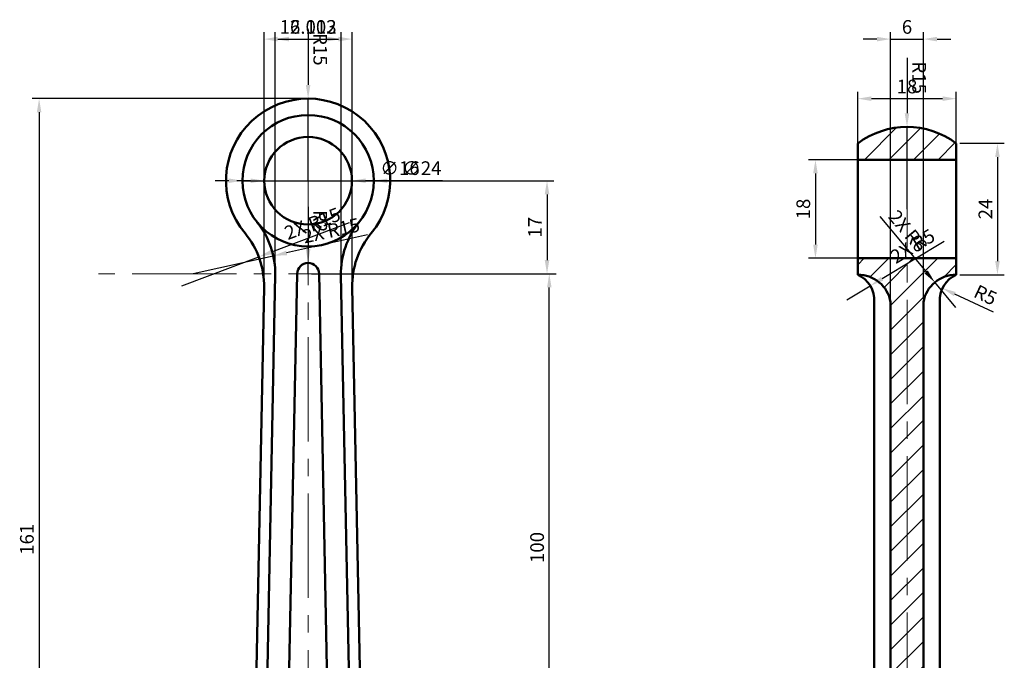
# Model space of a CAD drawing. Units: millimetres. Extents: x 2995 to 3180, y 2734 to 2968.
# Tile 3 of 3: x 2995 to 3175, y 2851 to 2968. Entities that reach past the tile are written whole.
import ezdxf

# ---------------------------------------------------------------- set-up
doc = ezdxf.new("R2010")
doc.units = ezdxf.units.MM
doc.linetypes.add('CENTER2', pattern=[28.575, 19.05, -3.175, 3.175, -3.175])
for name, color, linetype, lineweight in [('M-CNTR', 1, 'CENTER2', 18), ('M-DIMS', 2, 'Continuous', 25), ('M-HATC', 8, 'Continuous', 18), ('M-OUTL', 7, 'Continuous', 50)]:
    doc.layers.add(name, color=color, linetype=linetype, lineweight=lineweight)
doc.styles.get("Standard").update_dxf_attribs({"font": 'arial.ttf'})
doc.dimstyles.new('ISO-25', dxfattribs={"dimtxt": 2.5, "dimasz": 2.5, "dimexe": 1.25, "dimexo": 0.625, "dimtad": 1, "dimtxsty": 'Standard', "dimcen": 2.5, "dimadec": 0, "dimazin": 0, "dimtfac": 1, "dimtmove": 0, "dimatfit": 3, "dimfxl": 1, "dimarcsym": 0})

# ---------------------------------------------------------------- blocks, each defined once
blk = doc.blocks.new('*D15')
at = {"layer": 'Defpoints', "color": 0, "transparency": 16777216}
for p in [(3049.54, 2921.77), (3091.59, 2921.77), (3047.54, 2821.77)]:
    blk.add_point(p, dxfattribs=at)
at = {"layer": 'M-DIMS', "color": 0, "lineweight": -2, "transparency": 16777216}
for p, q in [((3050.17, 2921.77), (3092.84, 2921.77)), ((3091.59, 2824.27), (3091.59, 2919.27)), ((3048.17, 2821.77), (3092.84, 2821.77))]:
    blk.add_line(p, q, dxfattribs=at)
at = {"layer": 'M-DIMS', "color": 0, "transparency": 16777216}
for points in [[(3091.18, 2919.27), (3092.01, 2919.27), (3091.59, 2921.77)], [(3091.18, 2824.27), (3092.01, 2824.27), (3091.59, 2821.77)]]:
    blk.add_solid(points, dxfattribs=at)
at = {"layer": 'M-DIMS', "color": 0, "transparency": 16777216, "insert": (3089.69, 2871.77), "char_height": 2.5, "attachment_point": 5, "rotation": 90}
blk.add_mtext('100', dxfattribs=at)
blk = doc.blocks.new('*D16')
at = {"layer": 'Defpoints', "color": 0, "transparency": 16777216}
for p in [(3047.54, 2938.77), (3047.54, 2921.77), (3091.18, 2921.77)]:
    blk.add_point(p, dxfattribs=at)
at = {"layer": 'M-DIMS', "color": 0, "lineweight": -2, "transparency": 16777216}
for p, q in [((3048.17, 2938.77), (3092.43, 2938.77)), ((3091.18, 2936.27), (3091.18, 2924.27)), ((3048.17, 2921.77), (3092.43, 2921.77))]:
    blk.add_line(p, q, dxfattribs=at)
at = {"layer": 'M-DIMS', "color": 0, "transparency": 16777216}
for points in [[(3090.76, 2936.27), (3091.6, 2936.27), (3091.18, 2938.77)], [(3090.76, 2924.27), (3091.6, 2924.27), (3091.18, 2921.77)]]:
    blk.add_solid(points, dxfattribs=at)
at = {"layer": 'M-DIMS', "color": 0, "transparency": 16777216, "insert": (3089.3, 2930.27), "char_height": 2.5, "attachment_point": 5, "rotation": 90}
blk.add_mtext('17', dxfattribs=at)
blk = doc.blocks.new('*D17')
at = {"layer": 'Defpoints', "color": 0, "transparency": 16777216}
for p in [(3165.93, 2942.6), (3140.21, 2924.6), (3165.93, 2924.6)]:
    blk.add_point(p, dxfattribs=at)
at = {"layer": 'M-DIMS', "color": 0, "lineweight": -2, "transparency": 16777216}
for p, q in [((3165.31, 2942.6), (3138.96, 2942.6)), ((3140.21, 2940.1), (3140.21, 2927.1)), ((3165.31, 2924.6), (3138.96, 2924.6))]:
    blk.add_line(p, q, dxfattribs=at)
at = {"layer": 'M-DIMS', "color": 0, "transparency": 16777216}
for points in [[(3139.79, 2940.1), (3140.62, 2940.1), (3140.21, 2942.6)], [(3139.79, 2927.1), (3140.62, 2927.1), (3140.21, 2924.6)]]:
    blk.add_solid(points, dxfattribs=at)
at = {"layer": 'M-DIMS', "color": 0, "transparency": 16777216, "insert": (3138.31, 2933.6), "char_height": 2.5, "attachment_point": 5, "rotation": 90}
blk.add_mtext('18', dxfattribs=at)
blk = doc.blocks.new('*D18')
at = {"layer": 'Defpoints', "color": 0, "transparency": 16777216}
for p in [(3165.93, 2945.6), (3165.93, 2921.6), (3173.45, 2921.6)]:
    blk.add_point(p, dxfattribs=at)
at = {"layer": 'M-DIMS', "color": 0, "lineweight": -2, "transparency": 16777216}
for p, q in [((3166.56, 2945.6), (3174.7, 2945.6)), ((3173.45, 2943.1), (3173.45, 2924.1)), ((3166.56, 2921.6), (3174.7, 2921.6))]:
    blk.add_line(p, q, dxfattribs=at)
at = {"layer": 'M-DIMS', "color": 0, "transparency": 16777216}
for points in [[(3173.03, 2943.1), (3173.87, 2943.1), (3173.45, 2945.6)], [(3173.03, 2924.1), (3173.87, 2924.1), (3173.45, 2921.6)]]:
    blk.add_solid(points, dxfattribs=at)
at = {"layer": 'M-DIMS', "color": 0, "transparency": 16777216, "insert": (3171.57, 2933.6), "char_height": 2.5, "attachment_point": 5, "rotation": 90}
blk.add_mtext('24', dxfattribs=at)
blk = doc.blocks.new('*D19')
at = {"layer": 'Defpoints', "color": 0, "transparency": 16777216}
for p in [(3165.93, 2953.76), (3147.93, 2942.6), (3165.93, 2942.6)]:
    blk.add_point(p, dxfattribs=at)
at = {"layer": 'M-DIMS', "color": 0, "lineweight": -2, "transparency": 16777216}
for p, q in [((3147.93, 2943.22), (3147.93, 2955.01)), ((3165.93, 2943.22), (3165.93, 2955.01)), ((3150.43, 2953.76), (3163.43, 2953.76))]:
    blk.add_line(p, q, dxfattribs=at)
at = {"layer": 'M-DIMS', "color": 0, "transparency": 16777216}
for points in [[(3150.43, 2954.18), (3150.43, 2953.34), (3147.93, 2953.76)], [(3163.43, 2954.18), (3163.43, 2953.34), (3165.93, 2953.76)]]:
    blk.add_solid(points, dxfattribs=at)
at = {"layer": 'M-DIMS', "color": 0, "transparency": 16777216, "insert": (3156.93, 2955.66), "char_height": 2.5, "attachment_point": 5}
blk.add_mtext('18', dxfattribs=at)
blk = doc.blocks.new('*D25')
at = {"layer": 'Defpoints', "color": 0, "transparency": 16777216}
for p in [(3163.39, 2919.13), (3167.91, 2917.01)]:
    blk.add_point(p, dxfattribs=at)
at = {"layer": 'M-DIMS', "color": 0, "lineweight": -2, "transparency": 16777216}
blk.add_line((3172.71, 2914.76), (3165.65, 2918.07), dxfattribs=at)
at = {"layer": 'M-DIMS', "color": 0, "transparency": 16777216}
blk.add_solid([(3165.83, 2918.45), (3165.47, 2917.69), (3163.39, 2919.13)], dxfattribs=at)
at = {"layer": 'M-DIMS', "color": 0, "transparency": 16777216, "insert": (3171.12, 2917.6), "char_height": 2.5, "attachment_point": 5, "rotation": 334.8621}
blk.add_mtext('R5', dxfattribs=at)
blk = doc.blocks.new('*D28')
at = {"layer": 'Defpoints', "color": 0, "transparency": 16777216}
for p in [(3047.54, 2953.77), (2998.41, 2792.77), (3017.54, 2792.77)]:
    blk.add_point(p, dxfattribs=at)
at = {"layer": 'M-DIMS', "color": 0, "lineweight": -2, "transparency": 16777216}
for p, q in [((3046.92, 2953.77), (2997.16, 2953.77)), ((2998.41, 2951.27), (2998.41, 2795.27)), ((3016.92, 2792.77), (2997.16, 2792.77))]:
    blk.add_line(p, q, dxfattribs=at)
at = {"layer": 'M-DIMS', "color": 0, "transparency": 16777216}
for points in [[(2997.99, 2951.27), (2998.82, 2951.27), (2998.41, 2953.77)], [(2997.99, 2795.27), (2998.82, 2795.27), (2998.41, 2792.77)]]:
    blk.add_solid(points, dxfattribs=at)
at = {"layer": 'M-DIMS', "color": 0, "transparency": 16777216, "insert": (2996.5, 2873.27), "char_height": 2.5, "attachment_point": 5, "rotation": 90}
blk.add_mtext('161', dxfattribs=at)
blk = doc.blocks.new('*D30')
at = {"layer": 'Defpoints', "color": 0, "transparency": 16777216}
for p in [(3053.55, 2964.64), (3041.54, 2921.5), (3053.55, 2921.5)]:
    blk.add_point(p, dxfattribs=at)
at = {"layer": 'M-DIMS', "color": 0, "lineweight": -2, "transparency": 16777216}
for p, q in [((3041.54, 2922.12), (3041.54, 2965.89)), ((3053.55, 2922.12), (3053.55, 2965.89)), ((3044.04, 2964.64), (3051.05, 2964.64))]:
    blk.add_line(p, q, dxfattribs=at)
at = {"layer": 'M-DIMS', "color": 0, "transparency": 16777216}
for points in [[(3044.04, 2965.06), (3044.04, 2964.22), (3041.54, 2964.64)], [(3051.05, 2965.06), (3051.05, 2964.22), (3053.55, 2964.64)]]:
    blk.add_solid(points, dxfattribs=at)
at = {"layer": 'M-DIMS', "color": 0, "transparency": 16777216, "insert": (3047.54, 2966.54), "char_height": 2.5, "attachment_point": 5}
blk.add_mtext('12.012', dxfattribs=at)
blk = doc.blocks.new('*D31')
at = {"layer": 'Defpoints', "color": 0, "transparency": 16777216}
for p in [(3055.59, 2964.64), (3039.49, 2919.26), (3055.59, 2919.26)]:
    blk.add_point(p, dxfattribs=at)
at = {"layer": 'M-DIMS', "color": 0, "lineweight": -2, "transparency": 16777216}
for p, q in [((3039.49, 2919.89), (3039.49, 2965.89)), ((3055.59, 2919.89), (3055.59, 2965.89)), ((3041.99, 2964.64), (3053.09, 2964.64))]:
    blk.add_line(p, q, dxfattribs=at)
at = {"layer": 'M-DIMS', "color": 0, "transparency": 16777216}
for points in [[(3041.99, 2965.06), (3041.99, 2964.22), (3039.49, 2964.64)], [(3053.09, 2965.06), (3053.09, 2964.22), (3055.59, 2964.64)]]:
    blk.add_solid(points, dxfattribs=at)
at = {"layer": 'M-DIMS', "color": 0, "transparency": 16777216, "insert": (3047.54, 2966.54), "char_height": 2.5, "attachment_point": 5}
blk.add_mtext('16.103', dxfattribs=at)
blk = doc.blocks.new('*D35')
at = {"layer": 'Defpoints', "color": 0, "transparency": 16777216}
for p in [(3150.93, 2916.6), (3162.93, 2916.6), (3162.93, 2735.39)]:
    blk.add_point(p, dxfattribs=at)
at = {"layer": 'M-DIMS', "color": 0, "lineweight": -2, "transparency": 16777216}
for p, q in [((3150.93, 2915.97), (3150.93, 2734.14)), ((3162.93, 2915.97), (3162.93, 2734.14)), ((3153.43, 2735.39), (3160.43, 2735.39))]:
    blk.add_line(p, q, dxfattribs=at)
at = {"layer": 'M-DIMS', "color": 0, "transparency": 16777216}
for points in [[(3153.43, 2735.81), (3153.43, 2734.98), (3150.93, 2735.39)], [(3160.43, 2735.81), (3160.43, 2734.98), (3162.93, 2735.39)]]:
    blk.add_solid(points, dxfattribs=at)
at = {"layer": 'M-DIMS', "color": 0, "transparency": 16777216, "insert": (3156.93, 2737.27), "char_height": 2.5, "attachment_point": 5}
blk.add_mtext('12', dxfattribs=at)
blk = doc.blocks.new('*D36')
at = {"layer": 'Defpoints', "color": 0, "transparency": 16777216}
for p in [(3159.93, 2964.64), (3153.93, 2916.6), (3159.93, 2916.6)]:
    blk.add_point(p, dxfattribs=at)
at = {"layer": 'M-DIMS', "color": 0, "lineweight": -2, "transparency": 16777216}
for p, q in [((3153.93, 2917.22), (3153.93, 2965.89)), ((3159.93, 2917.22), (3159.93, 2965.89)), ((3151.43, 2964.64), (3148.93, 2964.64)), ((3153.93, 2964.64), (3159.93, 2964.64)), ((3162.43, 2964.64), (3164.93, 2964.64))]:
    blk.add_line(p, q, dxfattribs=at)
at = {"layer": 'M-DIMS', "color": 0, "transparency": 16777216}
for points in [[(3151.43, 2965.06), (3151.43, 2964.22), (3153.93, 2964.64)], [(3162.43, 2965.06), (3162.43, 2964.22), (3159.93, 2964.64)]]:
    blk.add_solid(points, dxfattribs=at)
at = {"layer": 'M-DIMS', "color": 0, "transparency": 16777216, "insert": (3156.93, 2966.54), "char_height": 2.5, "attachment_point": 5}
blk.add_mtext('6', dxfattribs=at)
blk = doc.blocks.new('*D37')
at = {"layer": 'Defpoints', "color": 0, "transparency": 16777216}
for p in [(3047.54, 2953.77), (3047.54, 2938.77)]:
    blk.add_point(p, dxfattribs=at)
at = {"layer": 'M-DIMS', "color": 0, "lineweight": -2, "transparency": 16777216}
for p, q in [((3047.54, 2966.39), (3047.54, 2956.27)), ((3047.54, 2938.77), (3047.54, 2953.77))]:
    blk.add_line(p, q, dxfattribs=at)
at = {"layer": 'M-DIMS', "color": 0, "transparency": 16777216}
blk.add_solid([(3047.96, 2956.27), (3047.12, 2956.27), (3047.54, 2953.77)], dxfattribs=at)
at = {"layer": 'M-DIMS', "color": 0, "transparency": 16777216, "insert": (3049.44, 2962.77), "char_height": 2.5, "attachment_point": 5, "rotation": 270.001}
blk.add_mtext('R15', dxfattribs=at)
blk = doc.blocks.new('*D38')
at = {"layer": 'Defpoints', "color": 0, "transparency": 16777216}
for p in [(3035.54, 2938.77), (3059.54, 2938.77)]:
    blk.add_point(p, dxfattribs=at)
at = {"layer": 'M-DIMS', "color": 0, "lineweight": -2, "transparency": 16777216}
for p, q in [((3033.04, 2938.77), (3030.54, 2938.77)), ((3035.54, 2938.77), (3059.54, 2938.77)), ((3072.08, 2938.77), (3062.04, 2938.77))]:
    blk.add_line(p, q, dxfattribs=at)
at = {"layer": 'M-DIMS', "color": 0, "transparency": 16777216}
for points in [[(3033.04, 2939.18), (3033.04, 2938.35), (3035.54, 2938.77)], [(3062.04, 2939.18), (3062.04, 2938.35), (3059.54, 2938.77)]]:
    blk.add_solid(points, dxfattribs=at)
at = {"layer": 'M-DIMS', "color": 0, "transparency": 16777216, "insert": (3068.31, 2940.74), "char_height": 2.5, "attachment_point": 5, "rotation": 359.999}
blk.add_mtext('∅24', dxfattribs=at)
blk = doc.blocks.new('*D39')
at = {"layer": 'Defpoints', "color": 0, "transparency": 16777216}
for p in [(3039.54, 2938.77), (3055.54, 2938.77)]:
    blk.add_point(p, dxfattribs=at)
at = {"layer": 'M-DIMS', "color": 0, "lineweight": -2, "transparency": 16777216}
for p, q in [((3037.04, 2938.77), (3034.54, 2938.77)), ((3039.54, 2938.77), (3055.54, 2938.77)), ((3068.09, 2938.77), (3058.04, 2938.77))]:
    blk.add_line(p, q, dxfattribs=at)
at = {"layer": 'M-DIMS', "color": 0, "transparency": 16777216}
for points in [[(3037.04, 2939.18), (3037.04, 2938.35), (3039.54, 2938.77)], [(3058.04, 2939.18), (3058.04, 2938.35), (3055.54, 2938.77)]]:
    blk.add_solid(points, dxfattribs=at)
at = {"layer": 'M-DIMS', "color": 0, "transparency": 16777216, "insert": (3064.32, 2940.74), "char_height": 2.5, "attachment_point": 5, "rotation": 359.9986}
blk.add_mtext('∅16', dxfattribs=at)
blk = doc.blocks.new('*D40')
at = {"layer": 'Defpoints', "color": 0, "transparency": 16777216}
for p in [(3038.53, 2924.86), (3024.49, 2919.56)]:
    blk.add_point(p, dxfattribs=at)
at = {"layer": 'M-DIMS', "color": 0, "lineweight": -2, "transparency": 16777216}
for p, q in [((3055.05, 2931.09), (3040.87, 2925.74)), ((3024.49, 2919.56), (3038.53, 2924.86))]:
    blk.add_line(p, q, dxfattribs=at)
at = {"layer": 'M-DIMS', "color": 0, "transparency": 16777216}
blk.add_solid([(3040.72, 2926.13), (3041.01, 2925.35), (3038.53, 2924.86)], dxfattribs=at)
at = {"layer": 'M-DIMS', "color": 0, "transparency": 16777216, "insert": (3048.45, 2930.64), "char_height": 2.5, "attachment_point": 5, "rotation": 20.6771}
blk.add_mtext('2X R15', dxfattribs=at)
blk = doc.blocks.new('*D41')
at = {"layer": 'Defpoints', "color": 0, "transparency": 16777216}
for p in [(3041.18, 2925.04), (3026.54, 2921.8)]:
    blk.add_point(p, dxfattribs=at)
at = {"layer": 'M-DIMS', "color": 0, "lineweight": -2, "transparency": 16777216}
for p, q in [((3058.42, 2928.86), (3043.62, 2925.58)), ((3026.54, 2921.8), (3041.18, 2925.04))]:
    blk.add_line(p, q, dxfattribs=at)
at = {"layer": 'M-DIMS', "color": 0, "transparency": 16777216}
blk.add_solid([(3043.53, 2925.99), (3043.71, 2925.17), (3041.18, 2925.04)], dxfattribs=at)
at = {"layer": 'M-DIMS', "color": 0, "transparency": 16777216, "insert": (3051.83, 2929.34), "char_height": 2.5, "attachment_point": 5, "rotation": 12.4787}
blk.add_mtext('2X R15', dxfattribs=at)
blk = doc.blocks.new('*D42')
at = {"layer": 'Defpoints', "color": 0, "transparency": 16777216}
for p in [(3047.54, 2923.77), (3047.54, 2921.77)]:
    blk.add_point(p, dxfattribs=at)
at = {"layer": 'M-DIMS', "color": 0, "lineweight": -2, "transparency": 16777216}
for p, q in [((3047.54, 2934.02), (3047.54, 2926.27)), ((3047.54, 2921.77), (3047.54, 2923.77))]:
    blk.add_line(p, q, dxfattribs=at)
at = {"layer": 'M-DIMS', "color": 0, "transparency": 16777216}
blk.add_solid([(3047.96, 2926.27), (3047.12, 2926.27), (3047.54, 2923.77)], dxfattribs=at)
at = {"layer": 'M-DIMS', "color": 0, "transparency": 16777216, "insert": (3049.42, 2931.39), "char_height": 2.5, "attachment_point": 5, "rotation": 270.0073}
blk.add_mtext('R2', dxfattribs=at)
blk = doc.blocks.new('*D51')
at = {"layer": 'Defpoints', "color": 0, "transparency": 16777216}
for p in [(3156.93, 2948.6), (3156.93, 2933.6)]:
    blk.add_point(p, dxfattribs=at)
at = {"layer": 'M-DIMS', "color": 0, "lineweight": -2, "transparency": 16777216}
for p, q in [((3156.93, 2961.22), (3156.93, 2951.1)), ((3156.93, 2933.6), (3156.93, 2948.6))]:
    blk.add_line(p, q, dxfattribs=at)
at = {"layer": 'M-DIMS', "color": 0, "transparency": 16777216}
blk.add_solid([(3157.35, 2951.1), (3156.51, 2951.1), (3156.93, 2948.6)], dxfattribs=at)
at = {"layer": 'M-DIMS', "color": 0, "transparency": 16777216, "insert": (3158.83, 2957.6), "char_height": 2.5, "attachment_point": 5, "rotation": 270.0015}
blk.add_mtext('R15', dxfattribs=at)
blk = doc.blocks.new('*D52')
at = {"layer": 'Defpoints', "color": 0, "transparency": 16777216}
for p in [(3162.01, 2920.21), (3165.85, 2915.6)]:
    blk.add_point(p, dxfattribs=at)
at = {"layer": 'M-DIMS', "color": 0, "lineweight": -2, "transparency": 16777216}
for p, q in [((3151.96, 2932.26), (3160.4, 2922.13)), ((3165.85, 2915.6), (3162.01, 2920.21))]:
    blk.add_line(p, q, dxfattribs=at)
at = {"layer": 'M-DIMS', "color": 0, "transparency": 16777216}
blk.add_solid([(3160.72, 2922.39), (3160.08, 2921.86), (3162.01, 2920.21)], dxfattribs=at)
at = {"layer": 'M-DIMS', "color": 0, "transparency": 16777216, "insert": (3156.84, 2929.37), "char_height": 2.5, "attachment_point": 5, "rotation": 309.8108}
blk.add_mtext('2X R6', dxfattribs=at)
blk = doc.blocks.new('*D53')
at = {"layer": 'Defpoints', "color": 0, "transparency": 16777216}
for p in [(3150.23, 2919.58), (3145.95, 2917.01)]:
    blk.add_point(p, dxfattribs=at)
at = {"layer": 'M-DIMS', "color": 0, "lineweight": -2, "transparency": 16777216}
for p, q in [((3163.7, 2927.67), (3152.38, 2920.87)), ((3145.95, 2917.01), (3150.23, 2919.58))]:
    blk.add_line(p, q, dxfattribs=at)
at = {"layer": 'M-DIMS', "color": 0, "transparency": 16777216}
blk.add_solid([(3152.16, 2921.23), (3152.59, 2920.51), (3150.23, 2919.58)], dxfattribs=at)
at = {"layer": 'M-DIMS', "color": 0, "transparency": 16777216, "insert": (3158.13, 2926.54), "char_height": 2.5, "attachment_point": 5, "rotation": 30.9917}
blk.add_mtext('2X R5', dxfattribs=at)

msp = doc.modelspace()

# ---------------------------------------------------------------- hatches: boundary and pattern name
at = {"layer": 'M-HATC'}
h = msp.add_hatch(dxfattribs=at)
h.set_pattern_fill('ANSI31', color=256)
h.paths.add_polyline_path([(3147.9304, 2945.5964), (3147.9304, 2942.5964), (3165.9304, 2942.5964), (3165.9304, 2945.5964, 0.33333333)])
h = msp.add_hatch(dxfattribs=at)
h.set_pattern_fill('ANSI31', color=256)
h.paths.add_polyline_path([(3147.9304, 2924.5964), (3147.9304, 2921.5964, -0.36997107), (3153.9304, 2916.5964), (3153.9304, 2819.5964, -0.41421356), (3148.9304, 2814.5964), (3142.9304, 2814.5964), (3142.9304, 2807.5964), (3170.9304, 2807.5964), (3170.9304, 2814.5964), (3164.9304, 2814.5964, -0.41421356), (3159.9304, 2819.5964), (3159.9304, 2916.5964, -0.36997107), (3165.9304, 2921.5964), (3165.9304, 2924.5964)])

# ---------------------------------------------------------------- linework, layer by layer
at = {"layer": 'M-CNTR'}
for p, q in [((3156.9304, 2945.5964), (3156.9304, 2810.5964)), ((3047.5413, 2938.7662), (3047.5413, 2821.7662)), ((3091.5923, 2921.7662), (3009.2802, 2921.7662))]:
    msp.add_line(p, q, dxfattribs=at)
at = {"layer": 'M-OUTL'}
for p, q in [((3147.9304, 2942.5964), (3147.9304, 2945.5964)), ((3165.9304, 2945.5964), (3165.9304, 2942.5964)), ((3147.9304, 2921.5964), (3147.9304, 2924.5964)), ((3165.9304, 2924.5964), (3165.9304, 2921.5964)), ((3041.5351, 2921.4996), (3039.5421, 2821.8462)), ((3045.5413, 2921.7662), (3043.5413, 2821.7662)), ((3049.5413, 2921.7662), (3051.5413, 2821.7662)), ((3053.5474, 2921.4996), (3055.5405, 2821.8462)), ((3039.49, 2919.2627), (3037.5425, 2821.8862)), ((3055.5925, 2919.2627), (3057.5401, 2821.8862)), ((3150.9304, 2822.5964), (3150.9304, 2916.5964)), ((3153.9304, 2916.5964), (3153.9304, 2819.5964)), ((3159.9304, 2916.5964), (3159.9304, 2819.5964)), ((3162.9304, 2916.5964), (3162.9304, 2822.5964))]:
    msp.add_line(p, q, dxfattribs=at)
msp.add_lwpolyline([(3147.9304, 2942.5964), (3165.9304, 2942.5964), (3165.9304, 2924.5964), (3147.9304, 2924.5964)], close=True, dxfattribs=at)
for radius in [12, 8]:
    msp.add_circle((3047.5413, 2938.7662), radius, dxfattribs=at)
for centre, radius, start, end in [((3047.5413, 2938.7662), 15, 320.1993, 219.8007), ((3156.9304, 2933.5964), 15, 53.130102, 126.869898), ((3026.5381, 2921.7995), 15, 358.854237, 38.931861), ((3068.5444, 2921.7995), 15, 141.068139, 181.145763), ((3024.493, 2919.5626), 15, 358.854237, 39.8007), ((3070.5895, 2919.5626), 15, 140.1993, 181.145763), ((3047.5413, 2921.7662), 2, 0, 180), ((3148.0142, 2915.597), 6, 9.588398, 90.80046), ((3145.9472, 2917.0065), 5, 355.295219, 66.632294), ((3165.8466, 2915.597), 6, 89.19954, 170.411602), ((3167.9135, 2917.0065), 5, 113.367706, 184.704781)]:
    msp.add_arc(centre, radius, start, end, dxfattribs=at)

# ---------------------------------------------------------------- dimensions: what is measured, and where the dimension line sits
at = {"layer": 'M-DIMS'}
for base, p1, p2, override, picture, middle in [((3055.59253, 2964.6412), (3039.48999, 2919.26269), (3055.59253, 2919.26269), {"dimdec": 3, "dimlfac": 1, "dimrnd": 0, "dimzin": 0, "dimdsep": 46, "dimlunit": 2}, '*D31', (3047.54126, 2966.54349)), ((3053.5474, 2964.6412), (3041.5351, 2921.4996), (3053.5474, 2921.4996), {"dimdec": 3, "dimlfac": 1, "dimrnd": 0, "dimzin": 0, "dimdsep": 46, "dimlunit": 2}, '*D30', (3047.5413, 2966.5426)), ((3159.9304, 2964.6412), (3153.9304, 2916.5964), (3159.9304, 2916.5964), {"dimdec": 0, "dimlfac": 1, "dimrnd": 0, "dimzin": 0, "dimdsep": 46, "dimlunit": 2}, '*D36', (3156.9304, 2966.5426)), ((3165.9304, 2953.7587), (3147.9304, 2942.5964), (3165.9304, 2942.5964), {"dimclrd": 0, "dimclre": 0, "dimclrt": 0}, '*D19', (3156.9304, 2955.6602)), ((3162.9304, 2735.3926), (3150.9304, 2916.5964), (3162.9304, 2916.5964), {"dimdec": 0, "dimlfac": 1, "dimrnd": 0, "dimzin": 0, "dimdsep": 46, "dimlunit": 2}, '*D35', (3156.9304, 2737.2727))]:
    dim = msp.add_linear_dim(base=base, p1=p1, p2=p2, dimstyle='ISO-25', override=override, dxfattribs=at)
    dim.commit()
    dim.dimension.update_dxf_attribs({"geometry": picture, "text_midpoint": middle})
for center, mpoint, override, picture, middle in [((3047.5413, 2938.7662), (3047.541, 2953.7662), {"dimdec": 0, "dimlfac": 1, "dimrnd": 0, "dimzin": 0, "dimdsep": 46, "dimlunit": 2}, '*D37', (3047.5408, 2962.7662)), ((3156.9304, 2933.5964), (3156.93, 2948.5964), {"dimdec": 0, "dimlfac": 1, "dimrnd": 0, "dimzin": 0, "dimdsep": 46, "dimlunit": 2}, '*D51', (3156.9298, 2957.5964)), ((3167.9135, 2917.0065), (3163.3871, 2919.1305), {"dimclrd": 0, "dimclre": 0, "dimclrt": 0}, '*D25', (3170.3126, 2915.8808))]:
    dim = msp.add_radius_dim(center=center, mpoint=mpoint, dimstyle='ISO-25', override=override, dxfattribs=at)
    dim.commit()
    dim.dimension.update_dxf_attribs({"geometry": picture, "text_midpoint": middle, "dimtype": 164})
for base, p1, p2, override, picture, middle in [((2998.4052, 2792.7662), (3047.5413, 2953.7662), (3017.5413, 2792.7662), {"dimdec": 0, "dimlfac": 1, "dimrnd": 0, "dimzin": 0, "dimdsep": 46, "dimlunit": 2}, '*D28', (2996.5038, 2873.2662)), ((3173.4516, 2921.5964), (3165.9304, 2945.5964), (3165.9304, 2921.5964), {"dimclrd": 0, "dimclre": 0, "dimclrt": 0}, '*D18', (3171.5715, 2933.5964)), ((3140.2074, 2924.5964), (3165.9304, 2942.5964), (3165.9304, 2924.5964), {"dimclrd": 0, "dimclre": 0, "dimclrt": 0}, '*D17', (3138.3059, 2933.5964)), ((3091.1806, 2921.7662), (3047.5413, 2938.7662), (3047.5413, 2921.7662), {"dimclrd": 0, "dimclre": 0, "dimclrt": 0}, '*D16', (3089.3005, 2930.2662)), ((3091.5923, 2921.7662), (3047.5413, 2821.7662), (3049.5413, 2921.7662), {"dimclrd": 0, "dimclre": 0, "dimclrt": 0}, '*D15', (3089.6908, 2871.7662))]:
    dim = msp.add_linear_dim(base=base, p1=p1, p2=p2, angle=90, dimstyle='ISO-25', override=override, dxfattribs=at)
    dim.commit()
    dim.dimension.update_dxf_attribs({"geometry": picture, "text_midpoint": middle})
for p1, p2, picture, middle in [((3035.5413, 2938.7664), (3059.5413, 2938.766), '*D38', (3068.3117, 2938.7659)), ((3039.5413, 2938.7664), (3055.5413, 2938.766), '*D39', (3064.316, 2938.7658))]:
    dim = msp.add_diameter_dim_2p(p1=p1, p2=p2, dimstyle='ISO-25', override={"dimdec": 0, "dimlfac": 1, "dimrnd": 0, "dimzin": 0, "dimdsep": 46, "dimlunit": 2}, dxfattribs=at)
    dim.commit()
    dim.dimension.update_dxf_attribs({"geometry": picture, "text_midpoint": middle})
for center, mpoint, picture, middle in [((3024.493, 2919.5626), (3038.5268, 2924.8591), '*D40', (3048.4541, 2930.6382)), ((3026.5381, 2921.7995), (3041.1838, 2925.0407), '*D41', (3051.8337, 2929.345)), ((3165.8466, 2915.597), (3162.005, 2920.206), '*D52', (3156.8409, 2929.3716)), ((3145.9472, 2917.0065), (3150.2334, 2919.5811), '*D53', (3158.1331, 2926.5442))]:
    dim = msp.add_radius_dim(center=center, mpoint=mpoint, text='2X <>', dimstyle='ISO-25', override={"dimdec": 0, "dimlfac": 1, "dimrnd": 0, "dimzin": 0, "dimdsep": 46, "dimlunit": 2}, dxfattribs=at)
    dim.commit()
    dim.dimension.update_dxf_attribs({"geometry": picture, "text_midpoint": middle})
dim = msp.add_radius_dim(center=(3047.5413, 2921.7662), mpoint=(3047.541, 2923.7662), dimstyle='ISO-25', override={"dimdec": 0, "dimlfac": 1, "dimrnd": 0, "dimzin": 0, "dimdsep": 46, "dimlunit": 2}, dxfattribs=at)
dim.commit()
dim.dimension.update_dxf_attribs({"geometry": '*D42', "text_midpoint": (3049.4201, 2931.3943)})

doc.saveas('drawing.dxf')
